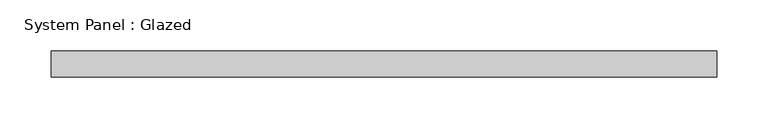
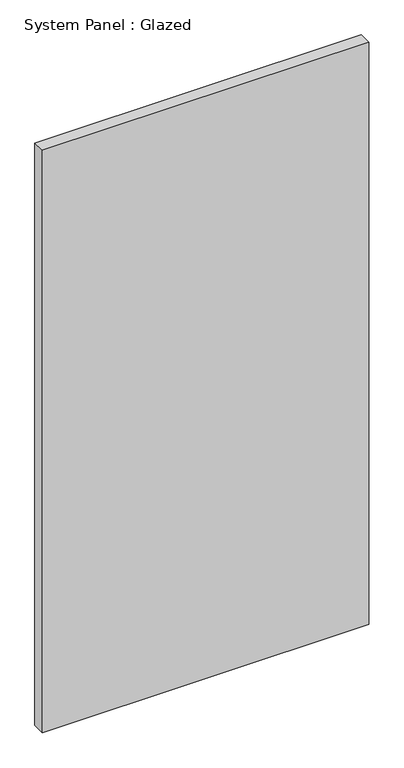
"""IFC4 building model written with IfcOpenShell, lengths in millimetres: plate geometry, System Panel : Glazed."""

from ifc_helpers import new_model, si_unit, origin, origin_with_axes, place, context, project, spatial, polyline, outline, extrude, source, transform, mapped, element, save


def system_panel_glazed_327d625d(model_context):
    return source(origin(), model_context, "Body", "SweptSolid", [
        extrude(outline(polyline([(323.85, 19.05), (-323.85, 19.05), (-323.85, 44.45), (323.85, 44.45), (323.85, 19.05)])), origin_with_axes(), (0.0, 0.0, 1.0), 1221.9870163),
    ])


if __name__ == "__main__":
    model = new_model("IFC4")
    model_context = context("Model", 3, world=origin())
    ifc_project = project(units=[si_unit("LENGTHUNIT", "METRE", prefix="MILLI")], contexts=[model_context])
    site = spatial("IfcSite", under=ifc_project)
    building = spatial("IfcBuilding", under=site)
    placement = place(None, origin())
    system_panel_glazed_shape = system_panel_glazed_327d625d(model_context)
    element("IfcPlate", 1, ObjectType="System Panel : Glazed", at=placement, inside=building, context=model_context, shape_type="MappedRepresentation", body=[
        mapped(system_panel_glazed_shape, transform((0.0, 0.0, 0.0), x_axis=(1.0, 0.0, 0.0), y_axis=(0.0, 1.0, 0.0), z_axis=(0.0, 0.0, 1.0))),
    ])
    save(model, "model.ifc")

# Revit data of these elements
# Type "System Panel : Glazed"
#   Construction Type Id = "GSP4R"
#   Analytic Construction = "1/8 in Pilkington single glazing"
#   Visual Light Transmittance = 0.9
#   Solar Heat Gain Coefficient = 0.86
#   Heat Transfer Coefficient (U) = 1.18115 BTU/(h·ft²·°F)
#   Define Thermal Properties by = 1
# Element 1 (IfcPlate, "System Panel : Glazed")
#   Materials on its faces: "Glass"
# Materials
#   "Glass": class "Glass", colour RGB 0 128 192, transparency 0.75, Description = "Soda Lime Glass", Cost = 0
